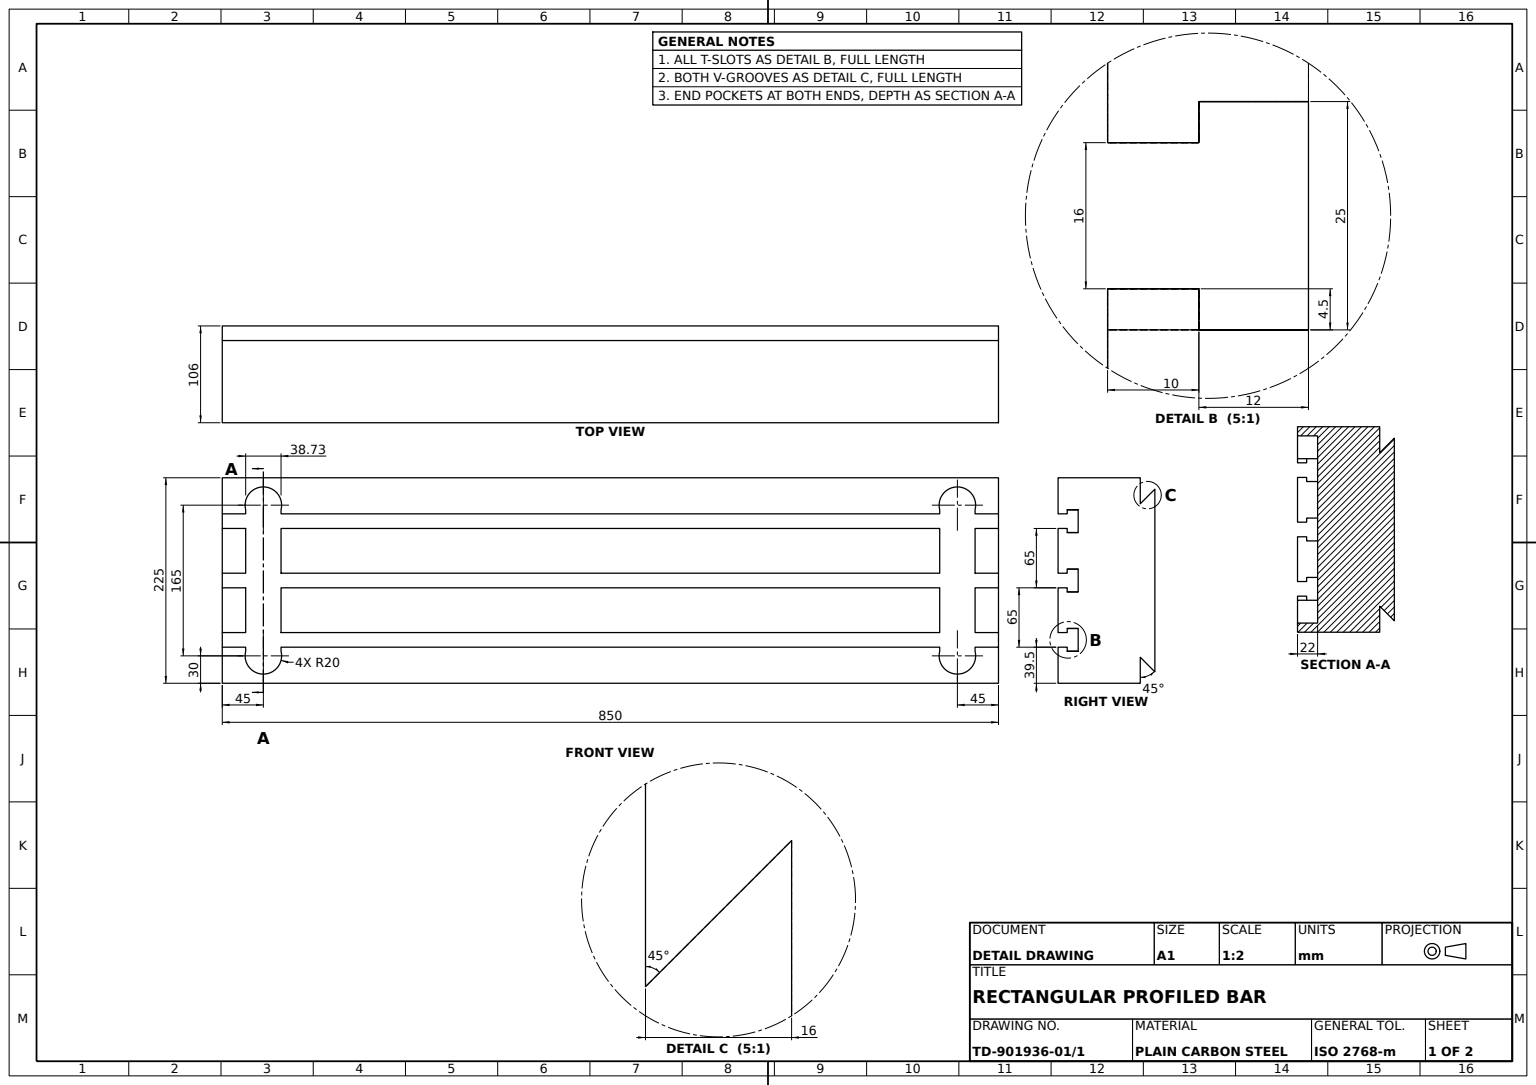
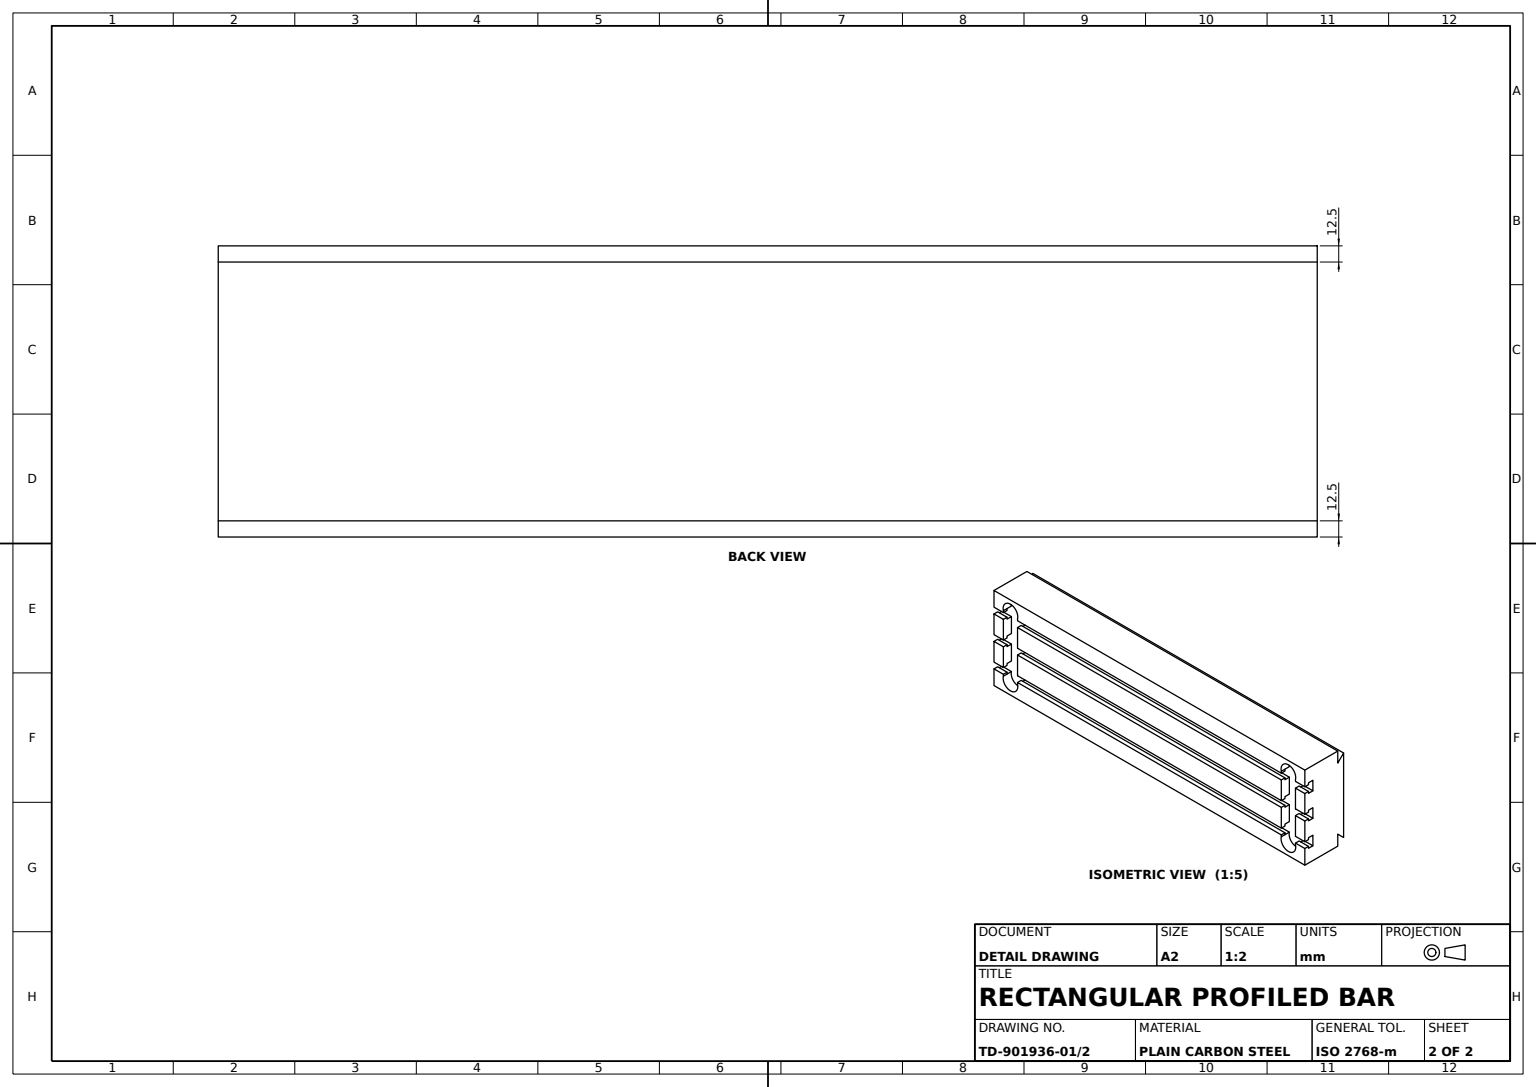
from build123d import *

# Parameters (mm, degrees)
BASE_BLOCK_PROFILE_W         = 850
BASE_BLOCK_PROFILE_H         = 225
BASE_BLOCK_850X225X106_DEPTH = 106
V_GROOVE_45DEG_DEPTH         = 864.939957404
T_SLOTS_2X_DEPTH             = 864.939957404
T_SLOT_END_POCKETS_REACH     = 454.236


with BuildPart() as part:
    # Base Block Profile → Base Block 850x225x106 (new body)
    with BuildSketch(Plane.XY):
        Rectangle(BASE_BLOCK_PROFILE_W, BASE_BLOCK_PROFILE_H)
    extrude(amount=BASE_BLOCK_850X225X106_DEPTH)

    # V-Groove Profile → V-Groove 45deg (cut, through all)
    with BuildSketch(Plane(origin=(425, 0, 0), x_dir=(0, 0, -1), z_dir=(1, 0, 0))):
        Polygon((-16, -112.5), (0, -112.5), (0, -100), (-16, -84), align=None)
        Polygon((-16, 84), (-16, 112.5), (0, 112.5), (0, 100), align=None)
    extrude(amount=-V_GROOVE_45DEG_DEPTH, mode=Mode.SUBTRACT)

    # T-Slots Profile → T-Slots 2x (cut, through all)
    with BuildSketch(Plane(origin=(425, 0, 0), x_dir=(0, 0, -1), z_dir=(1, 0, 0))):
        Polygon((-96, -12.5), (-84, -12.5), (-84, 12.5), (-96, 12.5), (-96, 8), (-106, 8), (-106, -8), (-96, -8), align=None)
        Polygon((-84, 77.5), (-84, 52.5), (-96, 52.5), (-96, 57), (-106, 57), (-106, 73), (-96, 73), (-96, 77.5), align=None)
        Polygon((-96, -77.5), (-84, -77.5), (-84, -52.5), (-96, -52.5), (-96, -57), (-106, -57), (-106, -73), (-96, -73), align=None)
    extrude(amount=-T_SLOTS_2X_DEPTH, mode=Mode.SUBTRACT)

    # T-Slot End Pockets: up to this face of the body (flat: up to its plane)
    t_slot_end_pockets_end = Plane(part.part.faces().sort_by_distance((0, 0, 84))[0])
    # T-Slot End Pockets Profile → T-Slot End Pockets (cut, up to the picked face)
    with BuildSketch(Plane.XY.offset(106), mode=Mode.PRIVATE) as t_slot_end_pockets_sk1:
        with BuildLine():
            Line((-399.363172475, -77.493249387), (-399.363172475, 77.493249387))
            ThreePointArc((-399.363172475, 77.493249387), (-380, 102.5), (-360.636827525, 77.493249387))
            Line((-360.636827525, 77.493249387), (-360.636827525, -77.493249387))
            ThreePointArc((-360.636827525, -77.493249387), (-380, -102.5), (-399.363172475, -77.493249387))
        make_face()
    t_slot_end_pockets_tool1 = split(extrude(t_slot_end_pockets_sk1.sketch, amount=-T_SLOT_END_POCKETS_REACH, mode=Mode.PRIVATE), bisect_by=t_slot_end_pockets_end, keep=Keep.BOTH, mode=Mode.PRIVATE)
    # T-Slot End Pockets Profile → T-Slot End Pockets (cut, up to the picked face)
    with BuildSketch(Plane.XY.offset(106), mode=Mode.PRIVATE) as t_slot_end_pockets_sk2:
        with BuildLine():
            Line((360.636827525, -77.493249387), (360.636827525, 77.493249387))
            ThreePointArc((360.636827525, 77.493249387), (380, 102.5), (399.363172475, 77.493249387))
            Line((399.363172475, 77.493249387), (399.363172475, -77.493249387))
            ThreePointArc((399.363172475, -77.493249387), (380, -102.5), (360.636827525, -77.493249387))
        make_face()
    t_slot_end_pockets_tool2 = split(extrude(t_slot_end_pockets_sk2.sketch, amount=-T_SLOT_END_POCKETS_REACH, mode=Mode.PRIVATE), bisect_by=t_slot_end_pockets_end, keep=Keep.BOTH, mode=Mode.PRIVATE)
    add(t_slot_end_pockets_tool1.solids().sort_by(Axis((-380, 0, 106), (0, 0, -1)))[0], mode=Mode.SUBTRACT)
    add(t_slot_end_pockets_tool2.solids().sort_by(Axis((380, 0, 106), (0, 0, -1)))[0], mode=Mode.SUBTRACT)


solid = part.part
